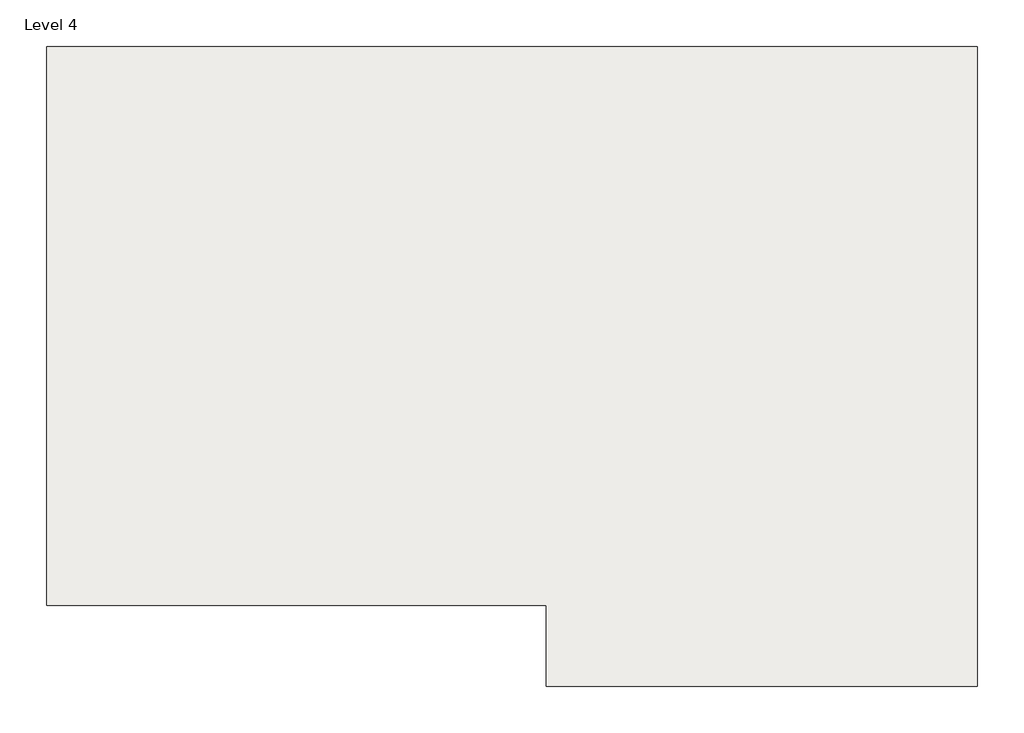
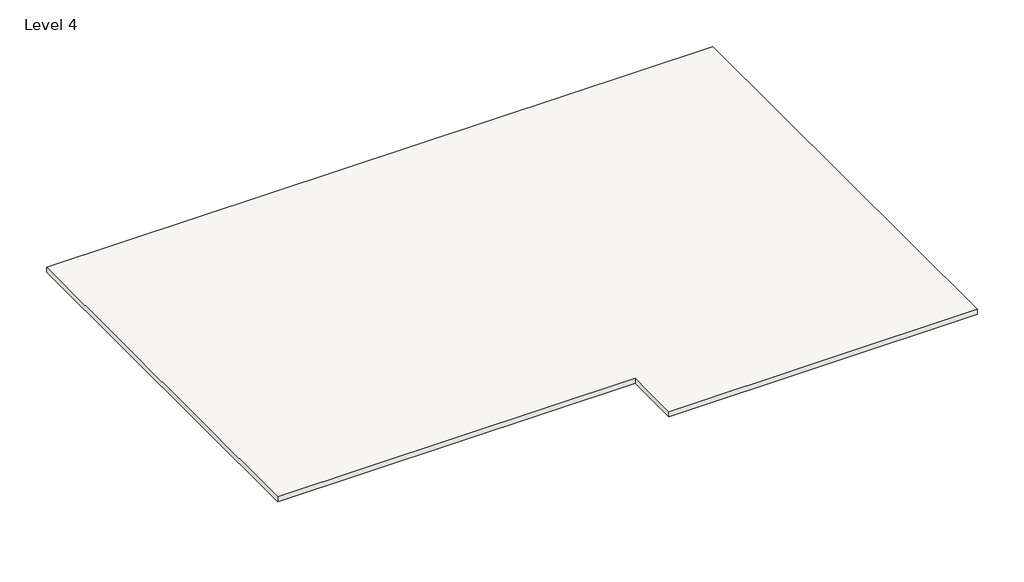
# One storey: 1 slab.
"""IFC4 building model written with IfcOpenShell, lengths in millimetres."""

from ifc_helpers import new_model, si_unit, frame, origin, place, context, project, spatial, polyline, outline, extrude, element, save

model = new_model("IFC4")

# Units and contexts
model_context = context("Model", 3, world=origin())
ifc_project = project(units=[si_unit("LENGTHUNIT", "METRE", prefix="MILLI")], contexts=[model_context])

# Site, building, storey
site = spatial("IfcSite", under=ifc_project)
building = spatial("IfcBuilding", under=site)
storey = spatial("IfcBuildingStorey", under=building, Name="Level 4", Elevation=7467.6)

# Slab
placement = place(None, origin())
element("IfcSlab", 1, ObjectType="6\" floor", at=placement, inside=storey, context=model_context, shape_type="SweptSolid", body=[
    extrude(outline(polyline([(-10470.5587801, -3005.0372669), (-10470.5587801, 8571.0127331), (8795.3412199, 8571.0127331), (8795.3412199, -4681.4372669), (-129.0484006, -4681.4372669), (-129.0484006, -3005.0372669), (-10470.5587801, -3005.0372669)])), frame((0.0, 0.0, 7467.6), z_axis=(0.0, 0.0, 1.0), x_axis=(1.0, 0.0, 0.0)), (0.0, 0.0, 1.0), 152.4),
])

save(model, "model.ifc")

# Revit data of these elements
# Type "6\" floor"
#   Assembly Code = "B1010"
#   Function = 0
#   Layers, outside or top first: 0' - 6" "Wall" (function 1)
# Element 1 (IfcSlab, "6\" floor")
#   built-in parameter 1001955 = -1.5708 (stored number, unit not read)
#   Height Offset From Level = 0' - 6"
#   Phase Created = New Construction
#   Materials on its faces: "Wall"
# Materials
#   "Wall": class "Generic", colour RGB 120 120 120, transparency 0, Cost = 0
